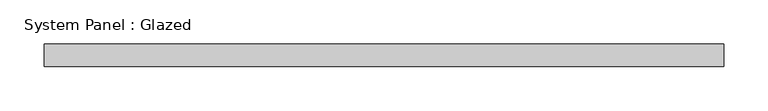
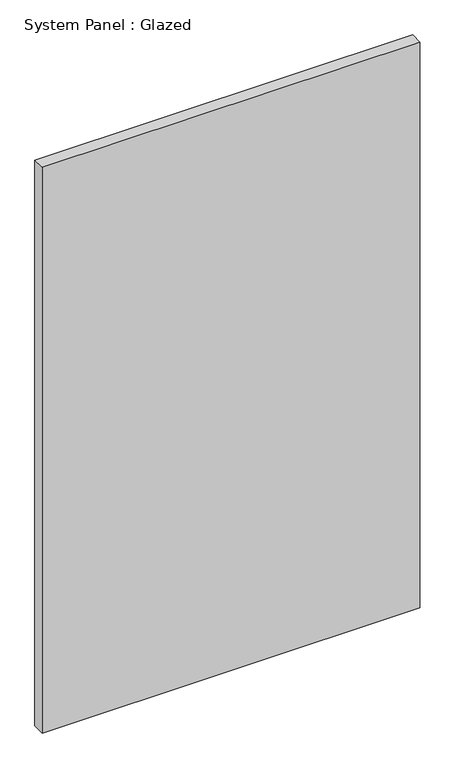
"""IFC4 building model written with IfcOpenShell, lengths in millimetres: plate geometry, System Panel : Glazed."""

from ifc_helpers import new_model, si_unit, origin, origin_with_axes, place, context, project, spatial, polyline, outline, extrude, source, transform, mapped, element, save


def system_panel_glazed_d0a3eec4(model_context):
    return source(origin(), model_context, "Body", "SweptSolid", [
        extrude(outline(polyline([(384.175, 19.05), (-384.175, 19.05), (-384.175, 44.45), (384.175, 44.45), (384.175, 19.05)])), origin_with_axes(), (0.0, 0.0, 1.0), 1216.8279521),
    ])


if __name__ == "__main__":
    model = new_model("IFC4")
    model_context = context("Model", 3, world=origin())
    ifc_project = project(units=[si_unit("LENGTHUNIT", "METRE", prefix="MILLI")], contexts=[model_context])
    site = spatial("IfcSite", under=ifc_project)
    building = spatial("IfcBuilding", under=site)
    placement = place(None, origin())
    system_panel_glazed_shape = system_panel_glazed_d0a3eec4(model_context)
    element("IfcPlate", 1, ObjectType="System Panel : Glazed", at=placement, inside=building, context=model_context, shape_type="MappedRepresentation", body=[
        mapped(system_panel_glazed_shape, transform((0.0, 0.0, 0.0), x_axis=(1.0, 0.0, 0.0), y_axis=(0.0, 1.0, 0.0), z_axis=(0.0, 0.0, 1.0))),
    ])
    save(model, "model.ifc")

# Revit data of these elements
# Type "System Panel : Glazed"
#   Construction Type Id = "GSP4R"
#   Analytic Construction = "1/8 in Pilkington single glazing"
#   Visual Light Transmittance = 0.9
#   Solar Heat Gain Coefficient = 0.86
#   Heat Transfer Coefficient (U) = 1.18115 BTU/(h·ft²·°F)
#   Define Thermal Properties by = 1
# Element 1 (IfcPlate, "System Panel : Glazed")
#   Materials on its faces: "Glass"
# Materials
#   "Glass": class "Glass", colour RGB 0 128 192, transparency 0.75, Description = "Soda Lime Glass", Cost = 0
